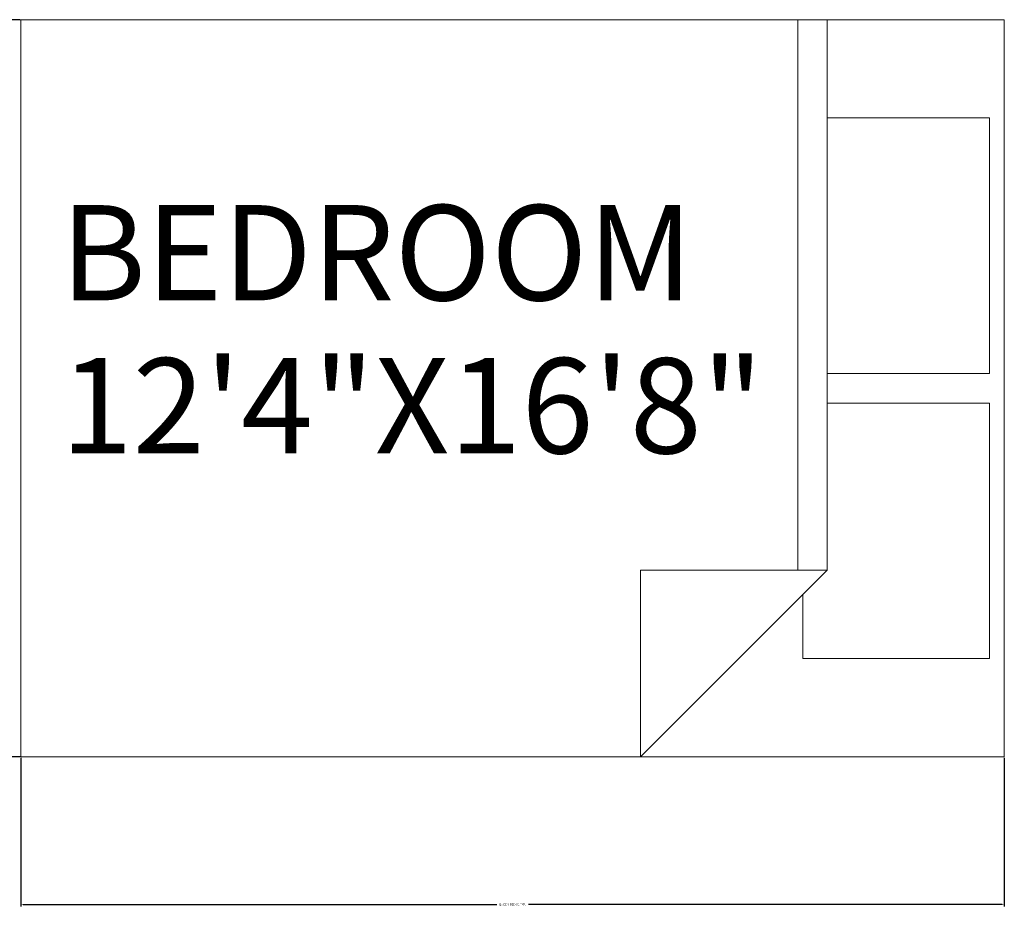
# Model space of a CAD drawing. Units: feet. Extents: x 2219 to 3039, y 1768 to 2369.
# Tile 14 of 16: x 2903 to 2984, y 2180 to 2253. Entities that reach past the tile are written whole.
import ezdxf

# ---------------------------------------------------------------- set-up
doc = ezdxf.new("R2010")
doc.units = ezdxf.units.FT
for name, color, linetype, lineweight in [('A-ANNO-DIMS', 2, 'Continuous', 18), ('A-AREA-IDEN', 7, 'Continuous', 18), ('A-FURN', 8, 'Continuous', 18)]:
    doc.layers.add(name, color=color, linetype=linetype, lineweight=lineweight)
doc.styles.get("Standard").update_dxf_attribs({"font": 'arial.ttf'})
doc.dimstyles.get("Standard").update_dxf_attribs({"dimtxt": 0.18, "dimasz": 0.18, "dimexe": 0.18, "dimexo": 0.0625, "dimgap": 0.09, "dimtad": 0, "dimtih": 1, "dimtoh": 1, "dimdec": 4, "dimzin": 0, "dimdsep": 46, "dimtxsty": 'Standard', "dimcen": 0.09, "dimadec": 0, "dimazin": 0, "dimtfac": 1, "dimtdec": 4, "dimtofl": 0, "dimtmove": 0, "dimatfit": 3, "dimfxl": 1, "dimtolj": 1, "dimtzin": 0, "dimarcsym": 0})

# ---------------------------------------------------------------- blocks, each defined once
blk = doc.blocks.new('Bed - Queen')
for p, q in [((0, -80.00003), (0, 0)), ((0, 0), (59.99999, 0)), ((59.99999, 0), (59.99999, -80.00003)), ((7.99999, -1.2), (28.79998, -1.2)), ((7.99999, -14.4), (7.99999, -1.2)), ((28.79998, -1.2), (28.79998, -14.4)), ((31.19999, -1.2), (51.99999, -1.2)), ((31.19999, -14.4), (31.19999, -1.2)), ((51.99999, -1.2), (51.99999, -16.4)), ((0, -14.4), (44.8, -14.4)), ((59.99999, -29.6), (44.8, -14.4)), ((44.8, -14.4), (44.8, -29.6)), ((44.8, -16.8), (0, -16.8)), ((51.99999, -16.4), (46.79936, -16.4)), ((44.8, -29.6), (59.99999, -29.6)), ((59.99999, -80.00003), (0, -80.00003))]:
    blk.add_line(p, q)
blk = doc.blocks.new('*D20')
at = {"layer": 'A-ANNO-DIMS', "color": 0, "lineweight": -2, "transparency": 16777216}
for p, q in [((2902.681, 2192.187), (2902.681, 2179.905)), ((2983.773, 2192.187), (2983.773, 2179.905)), ((2902.861, 2180.085), (2941.924, 2180.085)), ((2983.593, 2180.085), (2944.53, 2180.085))]:
    blk.add_line(p, q, dxfattribs=at)
at = {"layer": 'A-ANNO-DIMS', "color": 0, "transparency": 16777216}
for points in [[(2902.861, 2180.115), (2902.861, 2180.055), (2902.681, 2180.085)], [(2983.593, 2180.115), (2983.593, 2180.055), (2983.773, 2180.085)]]:
    blk.add_solid(points, dxfattribs=at)
at = {"layer": 'Defpoints', "color": 0, "transparency": 16777216}
for p in [(2902.681, 2192.249), (2983.773, 2192.249), (2983.773, 2180.085)]:
    blk.add_point(p, dxfattribs=at)
at = {"layer": 'A-ANNO-DIMS', "color": 0, "transparency": 16777216, "insert": (2943.227, 2180.085), "char_height": 0.18, "attachment_point": 5}
blk.add_mtext('\\A1;QUEEN BED 81 TYP.', dxfattribs=at)
blk = doc.blocks.new('*D21')
at = {"layer": 'A-ANNO-DIMS', "color": 0, "lineweight": -2, "transparency": 16777216}
for p, q in [((2902.619, 2253.068), (2890.337, 2253.068)), ((2890.517, 2252.888), (2890.517, 2222.841)), ((2890.517, 2192.429), (2890.517, 2222.477)), ((2902.619, 2192.249), (2890.337, 2192.249))]:
    blk.add_line(p, q, dxfattribs=at)
at = {"layer": 'A-ANNO-DIMS', "color": 0, "transparency": 16777216}
for points in [[(2890.487, 2252.888), (2890.547, 2252.888), (2890.517, 2253.068)], [(2890.487, 2192.429), (2890.547, 2192.429), (2890.517, 2192.249)]]:
    blk.add_solid(points, dxfattribs=at)
at = {"layer": 'Defpoints', "color": 0, "transparency": 16777216}
for p in [(2902.681, 2253.068), (2890.517, 2192.249), (2902.681, 2192.249)]:
    blk.add_point(p, dxfattribs=at)
at = {"layer": 'A-ANNO-DIMS', "color": 0, "transparency": 16777216, "insert": (2890.517, 2222.659), "char_height": 0.18, "attachment_point": 5}
blk.add_mtext('\\A1;61 TYP.', dxfattribs=at)

msp = doc.modelspace()

# ---------------------------------------------------------------- block references
at = {"layer": 'A-FURN', "xscale": 1.013648725183241, "yscale": 1.013648725183241, "zscale": 1.013648725183241, "rotation": 270}
msp.add_blockref('Bed - Queen', (2983.773, 2253.068), dxfattribs=at)

# ---------------------------------------------------------------- texts
at = {"layer": 'A-AREA-IDEN'}
for s, height, p in [('BEDROOM', 7.8584, (2905.95, 2229.916)), ('12\'4"X16\'8"', 7.85838, (2905.95, 2217.292))]:
    msp.add_text(s, height=height, dxfattribs=at).set_placement(p)

# ---------------------------------------------------------------- dimensions: what is measured, and where the dimension line sits
at = {"layer": 'A-ANNO-DIMS'}
dim = msp.add_linear_dim(base=(2890.517, 2192.249), p1=(2902.681, 2253.068), p2=(2902.681, 2192.249), angle=270, text='<> TYP.', dimstyle='Standard', override={"dimdec": 0, "dimlfac": 1, "dimrnd": 0, "dimzin": 0, "dimdsep": 46, "dimlunit": 2}, dxfattribs=at)
dim.commit()
dim.dimension.update_dxf_attribs({"geometry": '*D21', "text_midpoint": (2890.517, 2222.659)})
dim = msp.add_linear_dim(base=(2983.773, 2180.085), p1=(2902.681, 2192.249), p2=(2983.773, 2192.249), text='QUEEN BED <> TYP.', dimstyle='Standard', override={"dimdec": 0, "dimlfac": 1, "dimrnd": 0, "dimzin": 0, "dimdsep": 46, "dimlunit": 2}, dxfattribs=at)
dim.commit()
dim.dimension.update_dxf_attribs({"geometry": '*D20', "text_midpoint": (2943.227, 2180.085)})

doc.saveas('drawing.dxf')
